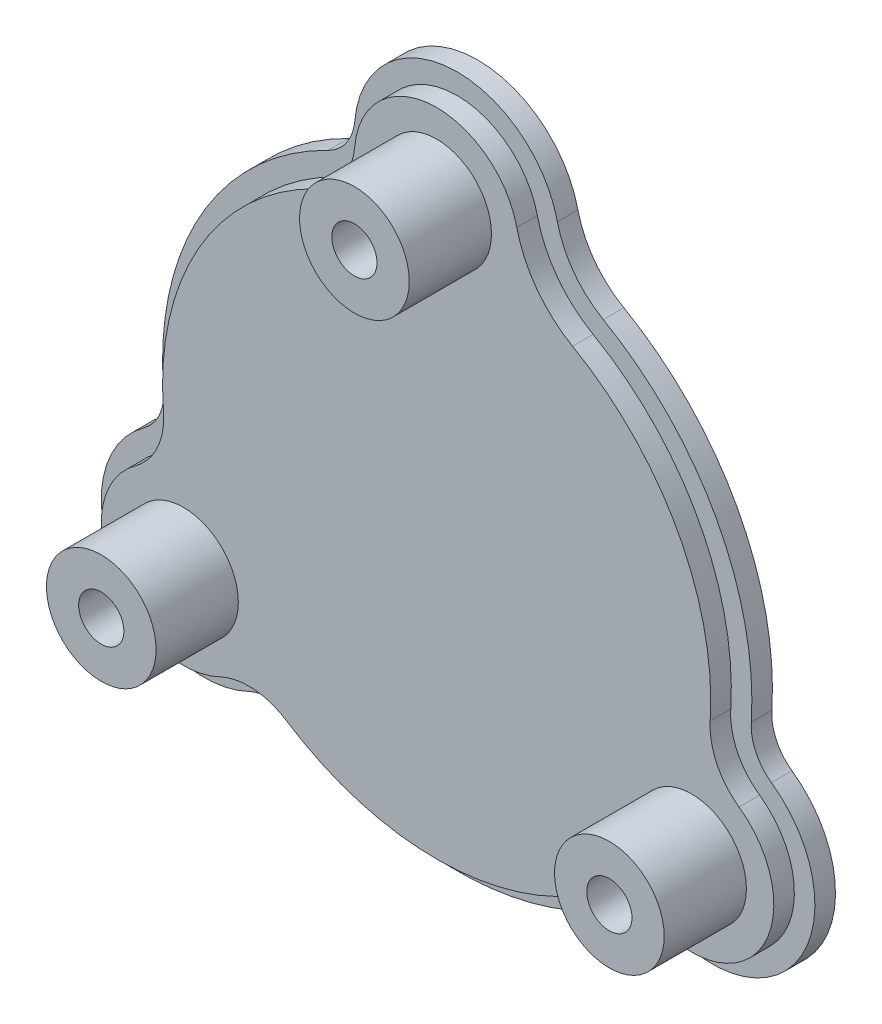
ISO-10303-21;
HEADER;
FILE_DESCRIPTION(('STEP AP214'),'2;1');
FILE_NAME('part.step','',(''),(''),'','','');
FILE_SCHEMA(('AUTOMOTIVE_DESIGN { 1 0 10303 214 1 1 1 1 }'));
ENDSEC;
DATA;
#1=APPLICATION_CONTEXT('core data for automotive mechanical design processes');
#2=APPLICATION_PROTOCOL_DEFINITION('international standard','automotive_design',2000,#1);
#3=PRODUCT_CONTEXT('',#1,'mechanical');
#4=PRODUCT('Part','Part','',(#3));
#5=PRODUCT_RELATED_PRODUCT_CATEGORY('part','',(#4));
#6=PRODUCT_DEFINITION_FORMATION('','',#4);
#7=PRODUCT_DEFINITION_CONTEXT('part definition',#1,'design');
#8=PRODUCT_DEFINITION('design','',#6,#7);
#9=PRODUCT_DEFINITION_SHAPE('','',#8);
#10=(LENGTH_UNIT() NAMED_UNIT(*) SI_UNIT(.MILLI.,.METRE.));
#11=(NAMED_UNIT(*) PLANE_ANGLE_UNIT() SI_UNIT($,.RADIAN.));
#12=(NAMED_UNIT(*) SI_UNIT($,.STERADIAN.) SOLID_ANGLE_UNIT());
#13=UNCERTAINTY_MEASURE_WITH_UNIT(LENGTH_MEASURE(1.E-05),#10,'distance_accuracy_value','');
#14=(GEOMETRIC_REPRESENTATION_CONTEXT(3) GLOBAL_UNCERTAINTY_ASSIGNED_CONTEXT((#13)) GLOBAL_UNIT_ASSIGNED_CONTEXT((#10,
#11,#12)) REPRESENTATION_CONTEXT('',''));
#15=CARTESIAN_POINT('',(0.,0.,0.));
#16=DIRECTION('',(0.,0.,1.));
#17=DIRECTION('',(1.,0.,0.));
#18=AXIS2_PLACEMENT_3D('',#15,#16,#17);
#19=CARTESIAN_POINT('',(-24.9125692180884,-2.08899376589599,3.));
#20=DIRECTION('',(0.,0.,1.));
#21=DIRECTION('',(1.,0.,0.));
#22=AXIS2_PLACEMENT_3D('',#19,#20,#21);
#23=PLANE('',#22);
#24=CARTESIAN_POINT('',(0.,0.,3.));
#25=DIRECTION('',(0.,0.,1.));
#26=DIRECTION('',(1.,0.,0.));
#27=AXIS2_PLACEMENT_3D('',#24,#25,#26);
#28=CIRCLE('',#27,43.);
#29=CARTESIAN_POINT('',(-18.8461534536892,38.65,3.));
#30=VERTEX_POINT('',#29);
#31=CARTESIAN_POINT('',(-42.8496190551121,-3.5930692773411,3.));
#32=VERTEX_POINT('',#31);
#33=EDGE_CURVE('E304',#30,#32,#28,.T.);
#34=ORIENTED_EDGE('',*,*,#33,.T.);
#35=CARTESIAN_POINT('',(-49.8251384361769,-4.17798753179198,3.));
#36=DIRECTION('',(0.,0.,-1.));
#37=DIRECTION('',(1.,0.,0.));
#38=AXIS2_PLACEMENT_3D('',#35,#36,#37);
#39=CIRCLE('',#38,7.);
#40=CARTESIAN_POINT('',(-45.7253382472528,-9.85175509936979,3.));
#41=VERTEX_POINT('',#40);
#42=EDGE_CURVE('E307',#32,#41,#39,.T.);
#43=ORIENTED_EDGE('',*,*,#42,.T.);
#44=CARTESIAN_POINT('',(-36.9400521281297,-22.0098284584651,3.));
#45=DIRECTION('',(0.,0.,1.));
#46=DIRECTION('',(1.,0.,0.));
#47=AXIS2_PLACEMENT_3D('',#44,#45,#46);
#48=CIRCLE('',#47,15.);
#49=CARTESIAN_POINT('',(-30.4295786984448,-35.5232934368253,3.));
#50=VERTEX_POINT('',#49);
#51=EDGE_CURVE('E309',#41,#50,#48,.T.);
#52=ORIENTED_EDGE('',*,*,#51,.T.);
#53=CARTESIAN_POINT('',(-27.3913577645918,-41.8295770933933,3.));
#54=DIRECTION('',(0.,0.,-1.));
#55=DIRECTION('',(1.,0.,0.));
#56=AXIS2_PLACEMENT_3D('',#53,#54,#55);
#57=CIRCLE('',#56,7.);
#58=CARTESIAN_POINT('',(-23.5565676775489,-35.9734363003183,3.));
#59=VERTEX_POINT('',#58);
#60=EDGE_CURVE('E315',#50,#59,#57,.T.);
#61=ORIENTED_EDGE('',*,*,#60,.T.);
#62=CARTESIAN_POINT('',(0.,0.,3.));
#63=DIRECTION('',(0.,0.,1.));
#64=DIRECTION('',(1.,0.,0.));
#65=AXIS2_PLACEMENT_3D('',#62,#63,#64);
#66=CIRCLE('',#65,43.);
#67=CARTESIAN_POINT('',(24.2998040125074,-35.4756187395474,3.));
#68=VERTEX_POINT('',#67);
#69=EDGE_CURVE('E314',#59,#68,#66,.T.);
#70=ORIENTED_EDGE('',*,*,#69,.T.);
#71=CARTESIAN_POINT('',(28.2555860610551,-41.25071946459,3.));
#72=DIRECTION('',(0.,0.,-1.));
#73=DIRECTION('',(1.,0.,0.));
#74=AXIS2_PLACEMENT_3D('',#71,#72,#73);
#75=CIRCLE('',#74,7.);
#76=CARTESIAN_POINT('',(31.1024364652992,-34.8557649865772,3.));
#77=VERTEX_POINT('',#76);
#78=EDGE_CURVE('E316',#68,#77,#75,.T.);
#79=ORIENTED_EDGE('',*,*,#78,.T.);
#80=CARTESIAN_POINT('',(37.2028301886792,-21.1522911051213,3.));
#81=DIRECTION('',(0.,0.,1.));
#82=DIRECTION('',(1.,0.,0.));
#83=AXIS2_PLACEMENT_3D('',#80,#81,#82);
#84=CIRCLE('',#83,15.);
#85=CARTESIAN_POINT('',(45.8589349502842,-8.90190946387765,3.));
#86=VERTEX_POINT('',#85);
#87=EDGE_CURVE('E318',#77,#86,#84,.T.);
#88=ORIENTED_EDGE('',*,*,#87,.T.);
#89=CARTESIAN_POINT('',(49.8984505056999,-3.18506469796396,3.));
#90=DIRECTION('',(0.,0.,-1.));
#91=DIRECTION('',(1.,0.,0.));
#92=AXIS2_PLACEMENT_3D('',#89,#90,#91);
#93=CIRCLE('',#92,7.);
#94=CARTESIAN_POINT('',(42.9126674349019,-2.739155640249,3.));
#95=VERTEX_POINT('',#94);
#96=EDGE_CURVE('E319',#86,#95,#93,.T.);
#97=ORIENTED_EDGE('',*,*,#96,.T.);
#98=CARTESIAN_POINT('',(0.,0.,3.));
#99=DIRECTION('',(0.,0.,1.));
#100=DIRECTION('',(1.,0.,0.));
#101=AXIS2_PLACEMENT_3D('',#98,#99,#100);
#102=CIRCLE('',#101,43.);
#103=CARTESIAN_POINT('',(21.320581007919,37.3421052631579,3.));
#104=VERTEX_POINT('',#103);
#105=EDGE_CURVE('E325',#95,#104,#102,.T.);
#106=ORIENTED_EDGE('',*,*,#105,.T.);
#107=CARTESIAN_POINT('',(28.2621655221252,49.5,3.));
#108=DIRECTION('',(0.,0.,-1.));
#109=DIRECTION('',(1.,0.,0.));
#110=AXIS2_PLACEMENT_3D('',#107,#108,#109);
#111=CIRCLE('',#110,14.);
#112=CARTESIAN_POINT('',(14.6183614769613,46.3620689655173,3.));
#113=VERTEX_POINT('',#112);
#114=EDGE_CURVE('E322',#104,#113,#111,.T.);
#115=ORIENTED_EDGE('',*,*,#114,.T.);
#116=CARTESIAN_POINT('',(0.,43.,3.));
#117=DIRECTION('',(0.,0.,1.));
#118=DIRECTION('',(1.,0.,0.));
#119=AXIS2_PLACEMENT_3D('',#116,#117,#118);
#120=CIRCLE('',#119,15.);
#121=CARTESIAN_POINT('',(-14.9414535837916,44.3239957716702,3.));
#122=VERTEX_POINT('',#121);
#123=EDGE_CURVE('E326',#113,#122,#120,.T.);
#124=ORIENTED_EDGE('',*,*,#123,.T.);
#125=CARTESIAN_POINT('',(-21.9141319228944,44.9418604651163,3.));
#126=DIRECTION('',(0.,0.,-1.));
#127=DIRECTION('',(1.,0.,0.));
#128=AXIS2_PLACEMENT_3D('',#125,#126,#127);
#129=CIRCLE('',#128,7.);
#130=EDGE_CURVE('E327',#122,#30,#129,.T.);
#131=ORIENTED_EDGE('',*,*,#130,.T.);
#132=EDGE_LOOP('',(#34,#43,#52,#61,#70,#79,#88,#97,#106,#115,#124,#131));
#133=FACE_BOUND('',#132,.T.);
#134=CARTESIAN_POINT('',(0.,0.,3.));
#135=DIRECTION('',(0.,0.,1.));
#136=DIRECTION('',(1.,0.,0.));
#137=AXIS2_PLACEMENT_3D('',#134,#135,#136);
#138=CIRCLE('',#137,40.);
#139=CARTESIAN_POINT('',(-17.5313055383155,35.953488372093,3.));
#140=VERTEX_POINT('',#139);
#141=CARTESIAN_POINT('',(-39.8601107489415,-3.34239002543356,3.));
#142=VERTEX_POINT('',#141);
#143=EDGE_CURVE('E218',#140,#142,#138,.T.);
#144=ORIENTED_EDGE('',*,*,#143,.F.);
#145=CARTESIAN_POINT('',(-21.9141319228944,44.9418604651163,3.));
#146=DIRECTION('',(0.,0.,1.));
#147=DIRECTION('',(1.,0.,0.));
#148=AXIS2_PLACEMENT_3D('',#145,#146,#147);
#149=CIRCLE('',#148,10.);
#150=CARTESIAN_POINT('',(-11.9531628670333,44.0591966173361,3.));
#151=VERTEX_POINT('',#150);
#152=EDGE_CURVE('E53',#140,#151,#149,.T.);
#153=ORIENTED_EDGE('',*,*,#152,.T.);
#154=CARTESIAN_POINT('',(0.,43.,3.));
#155=DIRECTION('',(0.,0.,1.));
#156=DIRECTION('',(1.,0.,0.));
#157=AXIS2_PLACEMENT_3D('',#154,#155,#156);
#158=CIRCLE('',#157,12.);
#159=CARTESIAN_POINT('',(11.694689181569,45.6896551724138,3.));
#160=VERTEX_POINT('',#159);
#161=EDGE_CURVE('E56',#160,#151,#158,.T.);
#162=ORIENTED_EDGE('',*,*,#161,.F.);
#163=CARTESIAN_POINT('',(28.2621655221252,49.5,3.));
#164=DIRECTION('',(0.,0.,1.));
#165=DIRECTION('',(1.,0.,0.));
#166=AXIS2_PLACEMENT_3D('',#163,#164,#165);
#167=CIRCLE('',#166,17.);
#168=CARTESIAN_POINT('',(19.8330986120176,34.7368421052632,3.));
#169=VERTEX_POINT('',#168);
#170=EDGE_CURVE('E251',#160,#169,#167,.T.);
#171=ORIENTED_EDGE('',*,*,#170,.T.);
#172=CARTESIAN_POINT('',(0.,0.,3.));
#173=DIRECTION('',(0.,0.,1.));
#174=DIRECTION('',(1.,0.,0.));
#175=AXIS2_PLACEMENT_3D('',#172,#173,#174);
#176=CIRCLE('',#175,40.);
#177=CARTESIAN_POINT('',(39.9187604045599,-2.54805175837117,3.));
#178=VERTEX_POINT('',#177);
#179=EDGE_CURVE('E254',#178,#169,#176,.T.);
#180=ORIENTED_EDGE('',*,*,#179,.F.);
#181=CARTESIAN_POINT('',(49.8984505056999,-3.18506469796396,3.));
#182=DIRECTION('',(0.,0.,1.));
#183=DIRECTION('',(1.,0.,0.));
#184=AXIS2_PLACEMENT_3D('',#181,#182,#183);
#185=CIRCLE('',#184,10.);
#186=CARTESIAN_POINT('',(44.1277139979632,-11.3519857921264,3.));
#187=VERTEX_POINT('',#186);
#188=EDGE_CURVE('E256',#178,#187,#185,.T.);
#189=ORIENTED_EDGE('',*,*,#188,.T.);
#190=CARTESIAN_POINT('',(37.2028301886792,-21.1522911051213,3.));
#191=DIRECTION('',(0.,0.,1.));
#192=DIRECTION('',(1.,0.,0.));
#193=AXIS2_PLACEMENT_3D('',#190,#191,#192);
#194=CIRCLE('',#193,12.);
#195=CARTESIAN_POINT('',(32.3225152099752,-32.115070210286,3.));
#196=VERTEX_POINT('',#195);
#197=EDGE_CURVE('E257',#196,#187,#194,.T.);
#198=ORIENTED_EDGE('',*,*,#197,.F.);
#199=CARTESIAN_POINT('',(28.2555860610551,-41.25071946459,3.));
#200=DIRECTION('',(0.,0.,1.));
#201=DIRECTION('',(1.,0.,0.));
#202=AXIS2_PLACEMENT_3D('',#199,#200,#201);
#203=CIRCLE('',#202,9.99999999999999);
#204=CARTESIAN_POINT('',(22.6044688488441,-33.000575571672,3.));
#205=VERTEX_POINT('',#204);
#206=EDGE_CURVE('E263',#196,#205,#203,.T.);
#207=ORIENTED_EDGE('',*,*,#206,.T.);
#208=CARTESIAN_POINT('',(0.,0.,3.));
#209=DIRECTION('',(0.,0.,1.));
#210=DIRECTION('',(1.,0.,0.));
#211=AXIS2_PLACEMENT_3D('',#208,#209,#210);
#212=CIRCLE('',#211,40.);
#213=CARTESIAN_POINT('',(-21.9130862116734,-33.4636616747147,3.));
#214=VERTEX_POINT('',#213);
#215=EDGE_CURVE('E264',#214,#205,#212,.T.);
#216=ORIENTED_EDGE('',*,*,#215,.F.);
#217=CARTESIAN_POINT('',(-27.3913577645918,-41.8295770933933,3.));
#218=DIRECTION('',(0.,0.,1.));
#219=DIRECTION('',(1.,0.,0.));
#220=AXIS2_PLACEMENT_3D('',#217,#218,#219);
#221=CIRCLE('',#220,10.);
#222=CARTESIAN_POINT('',(-31.7316733843817,-32.8206004411532,3.));
#223=VERTEX_POINT('',#222);
#224=EDGE_CURVE('E268',#214,#223,#221,.T.);
#225=ORIENTED_EDGE('',*,*,#224,.T.);
#226=CARTESIAN_POINT('',(-36.9400521281297,-22.0098284584651,3.));
#227=DIRECTION('',(0.,0.,1.));
#228=DIRECTION('',(1.,0.,0.));
#229=AXIS2_PLACEMENT_3D('',#226,#227,#228);
#230=CIRCLE('',#229,12.);
#231=CARTESIAN_POINT('',(-43.9682810234281,-12.2833697711889,3.));
#232=VERTEX_POINT('',#231);
#233=EDGE_CURVE('E269',#232,#223,#230,.T.);
#234=ORIENTED_EDGE('',*,*,#233,.F.);
#235=CARTESIAN_POINT('',(-49.8251384361769,-4.17798753179198,3.));
#236=DIRECTION('',(0.,0.,1.));
#237=DIRECTION('',(1.,0.,0.));
#238=AXIS2_PLACEMENT_3D('',#235,#236,#237);
#239=CIRCLE('',#238,10.);
#240=EDGE_CURVE('E225',#232,#142,#239,.T.);
#241=ORIENTED_EDGE('',*,*,#240,.T.);
#242=EDGE_LOOP('',(#144,#153,#162,#171,#180,#189,#198,#207,#216,#225,#234,#241));
#243=FACE_BOUND('',#242,.T.);
#244=ADVANCED_FACE('F39',(#133,#243),#23,.T.);
#245=CARTESIAN_POINT('',(0.,0.,3.));
#246=DIRECTION('',(0.,0.,-1.));
#247=DIRECTION('',(-1.,0.,0.));
#248=AXIS2_PLACEMENT_3D('',#245,#246,#247);
#249=CYLINDRICAL_SURFACE('',#248,43.);
#250=CARTESIAN_POINT('',(0.,0.,0.));
#251=DIRECTION('',(0.,0.,1.));
#252=DIRECTION('',(1.,0.,0.));
#253=AXIS2_PLACEMENT_3D('',#250,#251,#252);
#254=CIRCLE('',#253,43.);
#255=CARTESIAN_POINT('',(-18.8461534536892,38.65,0.));
#256=VERTEX_POINT('',#255);
#257=CARTESIAN_POINT('',(-42.8496190551121,-3.5930692773411,0.));
#258=VERTEX_POINT('',#257);
#259=EDGE_CURVE('E274',#256,#258,#254,.T.);
#260=ORIENTED_EDGE('',*,*,#259,.T.);
#261=DIRECTION('',(0.,0.,-1.));
#262=VECTOR('',#261,1.);
#263=CARTESIAN_POINT('',(-42.8496190551121,-3.5930692773411,3.));
#264=LINE('',#263,#262);
#265=EDGE_CURVE('E11',#32,#258,#264,.T.);
#266=ORIENTED_EDGE('',*,*,#265,.F.);
#267=ORIENTED_EDGE('',*,*,#33,.F.);
#268=DIRECTION('',(0.,0.,-1.));
#269=VECTOR('',#268,1.);
#270=CARTESIAN_POINT('',(-18.8461534536892,38.65,3.));
#271=LINE('',#270,#269);
#272=EDGE_CURVE('E329',#30,#256,#271,.T.);
#273=ORIENTED_EDGE('',*,*,#272,.T.);
#274=EDGE_LOOP('',(#260,#266,#267,#273));
#275=FACE_BOUND('',#274,.T.);
#276=ADVANCED_FACE('F41',(#275),#249,.T.);
#277=CARTESIAN_POINT('',(-49.8251384361769,-4.17798753179198,3.));
#278=DIRECTION('',(0.,0.,-1.));
#279=DIRECTION('',(-1.,0.,0.));
#280=AXIS2_PLACEMENT_3D('',#277,#278,#279);
#281=CYLINDRICAL_SURFACE('',#280,7.);
#282=CARTESIAN_POINT('',(-49.8251384361769,-4.17798753179198,0.));
#283=DIRECTION('',(0.,0.,-1.));
#284=DIRECTION('',(1.,0.,0.));
#285=AXIS2_PLACEMENT_3D('',#282,#283,#284);
#286=CIRCLE('',#285,7.);
#287=CARTESIAN_POINT('',(-45.7253382472528,-9.85175509936979,0.));
#288=VERTEX_POINT('',#287);
#289=EDGE_CURVE('E334',#258,#288,#286,.T.);
#290=ORIENTED_EDGE('',*,*,#289,.T.);
#291=DIRECTION('',(0.,0.,-1.));
#292=VECTOR('',#291,1.);
#293=CARTESIAN_POINT('',(-45.7253382472528,-9.85175509936979,3.));
#294=LINE('',#293,#292);
#295=EDGE_CURVE('E50',#41,#288,#294,.T.);
#296=ORIENTED_EDGE('',*,*,#295,.F.);
#297=ORIENTED_EDGE('',*,*,#42,.F.);
#298=ORIENTED_EDGE('',*,*,#265,.T.);
#299=EDGE_LOOP('',(#290,#296,#297,#298));
#300=FACE_BOUND('',#299,.T.);
#301=ADVANCED_FACE('F408',(#300),#281,.F.);
#302=CARTESIAN_POINT('',(-36.9400521281297,-22.0098284584651,3.));
#303=DIRECTION('',(0.,0.,-1.));
#304=DIRECTION('',(-1.,0.,0.));
#305=AXIS2_PLACEMENT_3D('',#302,#303,#304);
#306=CYLINDRICAL_SURFACE('',#305,15.);
#307=CARTESIAN_POINT('',(-36.9400521281297,-22.0098284584651,0.));
#308=DIRECTION('',(0.,0.,1.));
#309=DIRECTION('',(1.,0.,0.));
#310=AXIS2_PLACEMENT_3D('',#307,#308,#309);
#311=CIRCLE('',#310,15.);
#312=CARTESIAN_POINT('',(-30.4295786984448,-35.5232934368253,0.));
#313=VERTEX_POINT('',#312);
#314=EDGE_CURVE('E333',#288,#313,#311,.T.);
#315=ORIENTED_EDGE('',*,*,#314,.T.);
#316=DIRECTION('',(0.,0.,-1.));
#317=VECTOR('',#316,1.);
#318=CARTESIAN_POINT('',(-30.4295786984448,-35.5232934368253,3.));
#319=LINE('',#318,#317);
#320=EDGE_CURVE('E379',#50,#313,#319,.T.);
#321=ORIENTED_EDGE('',*,*,#320,.F.);
#322=ORIENTED_EDGE('',*,*,#51,.F.);
#323=ORIENTED_EDGE('',*,*,#295,.T.);
#324=EDGE_LOOP('',(#315,#321,#322,#323));
#325=FACE_BOUND('',#324,.T.);
#326=ADVANCED_FACE('F390',(#325),#306,.T.);
#327=CARTESIAN_POINT('',(-27.3913577645918,-41.8295770933933,3.));
#328=DIRECTION('',(0.,0.,-1.));
#329=DIRECTION('',(-1.,0.,0.));
#330=AXIS2_PLACEMENT_3D('',#327,#328,#329);
#331=CYLINDRICAL_SURFACE('',#330,7.);
#332=CARTESIAN_POINT('',(-27.3913577645918,-41.8295770933933,0.));
#333=DIRECTION('',(0.,0.,-1.));
#334=DIRECTION('',(1.,0.,0.));
#335=AXIS2_PLACEMENT_3D('',#332,#333,#334);
#336=CIRCLE('',#335,7.);
#337=CARTESIAN_POINT('',(-23.5565676775489,-35.9734363003183,0.));
#338=VERTEX_POINT('',#337);
#339=EDGE_CURVE('E336',#313,#338,#336,.T.);
#340=ORIENTED_EDGE('',*,*,#339,.T.);
#341=DIRECTION('',(0.,0.,-1.));
#342=VECTOR('',#341,1.);
#343=CARTESIAN_POINT('',(-23.5565676775489,-35.9734363003183,3.));
#344=LINE('',#343,#342);
#345=EDGE_CURVE('E380',#59,#338,#344,.T.);
#346=ORIENTED_EDGE('',*,*,#345,.F.);
#347=ORIENTED_EDGE('',*,*,#60,.F.);
#348=ORIENTED_EDGE('',*,*,#320,.T.);
#349=EDGE_LOOP('',(#340,#346,#347,#348));
#350=FACE_BOUND('',#349,.T.);
#351=ADVANCED_FACE('F396',(#350),#331,.F.);
#352=CARTESIAN_POINT('',(0.,0.,3.));
#353=DIRECTION('',(0.,0.,-1.));
#354=DIRECTION('',(-1.,0.,0.));
#355=AXIS2_PLACEMENT_3D('',#352,#353,#354);
#356=CYLINDRICAL_SURFACE('',#355,43.);
#357=CARTESIAN_POINT('',(0.,0.,0.));
#358=DIRECTION('',(0.,0.,1.));
#359=DIRECTION('',(1.,0.,0.));
#360=AXIS2_PLACEMENT_3D('',#357,#358,#359);
#361=CIRCLE('',#360,43.);
#362=CARTESIAN_POINT('',(24.2998040125074,-35.4756187395474,0.));
#363=VERTEX_POINT('',#362);
#364=EDGE_CURVE('E338',#338,#363,#361,.T.);
#365=ORIENTED_EDGE('',*,*,#364,.T.);
#366=DIRECTION('',(0.,0.,-1.));
#367=VECTOR('',#366,1.);
#368=CARTESIAN_POINT('',(24.2998040125074,-35.4756187395474,3.));
#369=LINE('',#368,#367);
#370=EDGE_CURVE('E372',#68,#363,#369,.T.);
#371=ORIENTED_EDGE('',*,*,#370,.F.);
#372=ORIENTED_EDGE('',*,*,#69,.F.);
#373=ORIENTED_EDGE('',*,*,#345,.T.);
#374=EDGE_LOOP('',(#365,#371,#372,#373));
#375=FACE_BOUND('',#374,.T.);
#376=ADVANCED_FACE('F405',(#375),#356,.T.);
#377=CARTESIAN_POINT('',(28.2555860610551,-41.25071946459,3.));
#378=DIRECTION('',(0.,0.,-1.));
#379=DIRECTION('',(-1.,0.,0.));
#380=AXIS2_PLACEMENT_3D('',#377,#378,#379);
#381=CYLINDRICAL_SURFACE('',#380,7.);
#382=CARTESIAN_POINT('',(28.2555860610551,-41.25071946459,0.));
#383=DIRECTION('',(0.,0.,-1.));
#384=DIRECTION('',(1.,0.,0.));
#385=AXIS2_PLACEMENT_3D('',#382,#383,#384);
#386=CIRCLE('',#385,7.);
#387=CARTESIAN_POINT('',(31.1024364652992,-34.8557649865772,0.));
#388=VERTEX_POINT('',#387);
#389=EDGE_CURVE('E343',#363,#388,#386,.T.);
#390=ORIENTED_EDGE('',*,*,#389,.T.);
#391=DIRECTION('',(0.,0.,-1.));
#392=VECTOR('',#391,1.);
#393=CARTESIAN_POINT('',(31.1024364652992,-34.8557649865772,3.));
#394=LINE('',#393,#392);
#395=EDGE_CURVE('E371',#77,#388,#394,.T.);
#396=ORIENTED_EDGE('',*,*,#395,.F.);
#397=ORIENTED_EDGE('',*,*,#78,.F.);
#398=ORIENTED_EDGE('',*,*,#370,.T.);
#399=EDGE_LOOP('',(#390,#396,#397,#398));
#400=FACE_BOUND('',#399,.T.);
#401=ADVANCED_FACE('F445',(#400),#381,.F.);
#402=CARTESIAN_POINT('',(37.2028301886792,-21.1522911051213,3.));
#403=DIRECTION('',(0.,0.,-1.));
#404=DIRECTION('',(-1.,0.,0.));
#405=AXIS2_PLACEMENT_3D('',#402,#403,#404);
#406=CYLINDRICAL_SURFACE('',#405,15.);
#407=CARTESIAN_POINT('',(37.2028301886792,-21.1522911051213,0.));
#408=DIRECTION('',(0.,0.,1.));
#409=DIRECTION('',(1.,0.,0.));
#410=AXIS2_PLACEMENT_3D('',#407,#408,#409);
#411=CIRCLE('',#410,15.);
#412=CARTESIAN_POINT('',(45.8589349502842,-8.90190946387765,0.));
#413=VERTEX_POINT('',#412);
#414=EDGE_CURVE('E341',#388,#413,#411,.T.);
#415=ORIENTED_EDGE('',*,*,#414,.T.);
#416=DIRECTION('',(0.,0.,-1.));
#417=VECTOR('',#416,1.);
#418=CARTESIAN_POINT('',(45.8589349502842,-8.90190946387765,3.));
#419=LINE('',#418,#417);
#420=EDGE_CURVE('E366',#86,#413,#419,.T.);
#421=ORIENTED_EDGE('',*,*,#420,.F.);
#422=ORIENTED_EDGE('',*,*,#87,.F.);
#423=ORIENTED_EDGE('',*,*,#395,.T.);
#424=EDGE_LOOP('',(#415,#421,#422,#423));
#425=FACE_BOUND('',#424,.T.);
#426=ADVANCED_FACE('F439',(#425),#406,.T.);
#427=CARTESIAN_POINT('',(49.8984505056999,-3.18506469796396,3.));
#428=DIRECTION('',(0.,0.,-1.));
#429=DIRECTION('',(-1.,0.,0.));
#430=AXIS2_PLACEMENT_3D('',#427,#428,#429);
#431=CYLINDRICAL_SURFACE('',#430,7.);
#432=CARTESIAN_POINT('',(49.8984505056999,-3.18506469796396,0.));
#433=DIRECTION('',(0.,0.,-1.));
#434=DIRECTION('',(1.,0.,0.));
#435=AXIS2_PLACEMENT_3D('',#432,#433,#434);
#436=CIRCLE('',#435,7.);
#437=CARTESIAN_POINT('',(42.9126674349019,-2.739155640249,0.));
#438=VERTEX_POINT('',#437);
#439=EDGE_CURVE('E342',#413,#438,#436,.T.);
#440=ORIENTED_EDGE('',*,*,#439,.T.);
#441=DIRECTION('',(0.,0.,-1.));
#442=VECTOR('',#441,1.);
#443=CARTESIAN_POINT('',(42.9126674349019,-2.739155640249,3.));
#444=LINE('',#443,#442);
#445=EDGE_CURVE('E364',#95,#438,#444,.T.);
#446=ORIENTED_EDGE('',*,*,#445,.F.);
#447=ORIENTED_EDGE('',*,*,#96,.F.);
#448=ORIENTED_EDGE('',*,*,#420,.T.);
#449=EDGE_LOOP('',(#440,#446,#447,#448));
#450=FACE_BOUND('',#449,.T.);
#451=ADVANCED_FACE('F436',(#450),#431,.F.);
#452=CARTESIAN_POINT('',(0.,0.,3.));
#453=DIRECTION('',(0.,0.,-1.));
#454=DIRECTION('',(-1.,0.,0.));
#455=AXIS2_PLACEMENT_3D('',#452,#453,#454);
#456=CYLINDRICAL_SURFACE('',#455,43.);
#457=CARTESIAN_POINT('',(0.,0.,0.));
#458=DIRECTION('',(0.,0.,1.));
#459=DIRECTION('',(1.,0.,0.));
#460=AXIS2_PLACEMENT_3D('',#457,#458,#459);
#461=CIRCLE('',#460,43.);
#462=CARTESIAN_POINT('',(21.320581007919,37.3421052631579,0.));
#463=VERTEX_POINT('',#462);
#464=EDGE_CURVE('E350',#438,#463,#461,.T.);
#465=ORIENTED_EDGE('',*,*,#464,.T.);
#466=DIRECTION('',(0.,0.,-1.));
#467=VECTOR('',#466,1.);
#468=CARTESIAN_POINT('',(21.320581007919,37.3421052631579,3.));
#469=LINE('',#468,#467);
#470=EDGE_CURVE('E362',#104,#463,#469,.T.);
#471=ORIENTED_EDGE('',*,*,#470,.F.);
#472=ORIENTED_EDGE('',*,*,#105,.F.);
#473=ORIENTED_EDGE('',*,*,#445,.T.);
#474=EDGE_LOOP('',(#465,#471,#472,#473));
#475=FACE_BOUND('',#474,.T.);
#476=ADVANCED_FACE('F431',(#475),#456,.T.);
#477=CARTESIAN_POINT('',(28.2621655221252,49.5,3.));
#478=DIRECTION('',(0.,0.,-1.));
#479=DIRECTION('',(-1.,0.,0.));
#480=AXIS2_PLACEMENT_3D('',#477,#478,#479);
#481=CYLINDRICAL_SURFACE('',#480,14.);
#482=CARTESIAN_POINT('',(28.2621655221252,49.5,0.));
#483=DIRECTION('',(0.,0.,-1.));
#484=DIRECTION('',(1.,0.,0.));
#485=AXIS2_PLACEMENT_3D('',#482,#483,#484);
#486=CIRCLE('',#485,14.);
#487=CARTESIAN_POINT('',(14.6183614769613,46.3620689655173,0.));
#488=VERTEX_POINT('',#487);
#489=EDGE_CURVE('E349',#463,#488,#486,.T.);
#490=ORIENTED_EDGE('',*,*,#489,.T.);
#491=DIRECTION('',(0.,0.,-1.));
#492=VECTOR('',#491,1.);
#493=CARTESIAN_POINT('',(14.6183614769613,46.3620689655173,3.));
#494=LINE('',#493,#492);
#495=EDGE_CURVE('E359',#113,#488,#494,.T.);
#496=ORIENTED_EDGE('',*,*,#495,.F.);
#497=ORIENTED_EDGE('',*,*,#114,.F.);
#498=ORIENTED_EDGE('',*,*,#470,.T.);
#499=EDGE_LOOP('',(#490,#496,#497,#498));
#500=FACE_BOUND('',#499,.T.);
#501=ADVANCED_FACE('F422',(#500),#481,.F.);
#502=CARTESIAN_POINT('',(0.,43.,3.));
#503=DIRECTION('',(0.,0.,-1.));
#504=DIRECTION('',(-1.,0.,0.));
#505=AXIS2_PLACEMENT_3D('',#502,#503,#504);
#506=CYLINDRICAL_SURFACE('',#505,15.);
#507=CARTESIAN_POINT('',(0.,43.,0.));
#508=DIRECTION('',(0.,0.,1.));
#509=DIRECTION('',(1.,0.,0.));
#510=AXIS2_PLACEMENT_3D('',#507,#508,#509);
#511=CIRCLE('',#510,15.);
#512=CARTESIAN_POINT('',(-14.9414535837916,44.3239957716702,0.));
#513=VERTEX_POINT('',#512);
#514=EDGE_CURVE('E354',#488,#513,#511,.T.);
#515=ORIENTED_EDGE('',*,*,#514,.T.);
#516=DIRECTION('',(0.,0.,-1.));
#517=VECTOR('',#516,1.);
#518=CARTESIAN_POINT('',(-14.9414535837916,44.3239957716702,3.));
#519=LINE('',#518,#517);
#520=EDGE_CURVE('E358',#122,#513,#519,.T.);
#521=ORIENTED_EDGE('',*,*,#520,.F.);
#522=ORIENTED_EDGE('',*,*,#123,.F.);
#523=ORIENTED_EDGE('',*,*,#495,.T.);
#524=EDGE_LOOP('',(#515,#521,#522,#523));
#525=FACE_BOUND('',#524,.T.);
#526=ADVANCED_FACE('F423',(#525),#506,.T.);
#527=CARTESIAN_POINT('',(-21.9141319228944,44.9418604651163,3.));
#528=DIRECTION('',(0.,0.,-1.));
#529=DIRECTION('',(-1.,0.,0.));
#530=AXIS2_PLACEMENT_3D('',#527,#528,#529);
#531=CYLINDRICAL_SURFACE('',#530,7.);
#532=CARTESIAN_POINT('',(-21.9141319228944,44.9418604651163,0.));
#533=DIRECTION('',(0.,0.,-1.));
#534=DIRECTION('',(1.,0.,0.));
#535=AXIS2_PLACEMENT_3D('',#532,#533,#534);
#536=CIRCLE('',#535,7.);
#537=EDGE_CURVE('E306',#513,#256,#536,.T.);
#538=ORIENTED_EDGE('',*,*,#537,.T.);
#539=ORIENTED_EDGE('',*,*,#272,.F.);
#540=ORIENTED_EDGE('',*,*,#130,.F.);
#541=ORIENTED_EDGE('',*,*,#520,.T.);
#542=EDGE_LOOP('',(#538,#539,#540,#541));
#543=FACE_BOUND('',#542,.T.);
#544=ADVANCED_FACE('F418',(#543),#531,.F.);
#545=CARTESIAN_POINT('',(-24.9125692180884,-2.08899376589599,0.));
#546=DIRECTION('',(0.,0.,1.));
#547=DIRECTION('',(1.,0.,0.));
#548=AXIS2_PLACEMENT_3D('',#545,#546,#547);
#549=PLANE('',#548);
#550=CARTESIAN_POINT('',(0.,43.,0.));
#551=DIRECTION('',(0.,0.,1.));
#552=DIRECTION('',(1.,0.,0.));
#553=AXIS2_PLACEMENT_3D('',#550,#551,#552);
#554=CIRCLE('',#553,3.3);
#555=CARTESIAN_POINT('',(3.3,43.,0.));
#556=VERTEX_POINT('',#555);
#557=EDGE_CURVE('E726',#556,#556,#554,.T.);
#558=ORIENTED_EDGE('',*,*,#557,.T.);
#559=EDGE_LOOP('',(#558));
#560=FACE_BOUND('',#559,.T.);
#561=CARTESIAN_POINT('',(37.2028301886792,-21.1522911051213,0.));
#562=DIRECTION('',(0.,0.,1.));
#563=DIRECTION('',(1.,0.,0.));
#564=AXIS2_PLACEMENT_3D('',#561,#562,#563);
#565=CIRCLE('',#564,3.3);
#566=CARTESIAN_POINT('',(40.5028301886792,-21.1522911051213,0.));
#567=VERTEX_POINT('',#566);
#568=EDGE_CURVE('E727',#567,#567,#565,.T.);
#569=ORIENTED_EDGE('',*,*,#568,.T.);
#570=EDGE_LOOP('',(#569));
#571=FACE_BOUND('',#570,.T.);
#572=CARTESIAN_POINT('',(-36.9400521281297,-22.0098284584651,0.));
#573=DIRECTION('',(0.,0.,1.));
#574=DIRECTION('',(1.,0.,0.));
#575=AXIS2_PLACEMENT_3D('',#572,#573,#574);
#576=CIRCLE('',#575,3.3);
#577=CARTESIAN_POINT('',(-33.6400521281297,-22.0098284584651,0.));
#578=VERTEX_POINT('',#577);
#579=EDGE_CURVE('E739',#578,#578,#576,.T.);
#580=ORIENTED_EDGE('',*,*,#579,.T.);
#581=EDGE_LOOP('',(#580));
#582=FACE_BOUND('',#581,.T.);
#583=ORIENTED_EDGE('',*,*,#259,.F.);
#584=ORIENTED_EDGE('',*,*,#537,.F.);
#585=ORIENTED_EDGE('',*,*,#514,.F.);
#586=ORIENTED_EDGE('',*,*,#489,.F.);
#587=ORIENTED_EDGE('',*,*,#464,.F.);
#588=ORIENTED_EDGE('',*,*,#439,.F.);
#589=ORIENTED_EDGE('',*,*,#414,.F.);
#590=ORIENTED_EDGE('',*,*,#389,.F.);
#591=ORIENTED_EDGE('',*,*,#364,.F.);
#592=ORIENTED_EDGE('',*,*,#339,.F.);
#593=ORIENTED_EDGE('',*,*,#314,.F.);
#594=ORIENTED_EDGE('',*,*,#289,.F.);
#595=EDGE_LOOP('',(#583,#584,#585,#586,#587,#588,#589,#590,#591,#592,#593,#594));
#596=FACE_BOUND('',#595,.T.);
#597=ADVANCED_FACE('F395',(#560,#571,#582,#596),#549,.F.);
#598=CARTESIAN_POINT('',(-21.9141319228944,44.9418604651163,6.));
#599=DIRECTION('',(0.,0.,-1.));
#600=DIRECTION('',(-1.,0.,0.));
#601=AXIS2_PLACEMENT_3D('',#598,#599,#600);
#602=CYLINDRICAL_SURFACE('',#601,10.);
#603=ORIENTED_EDGE('',*,*,#152,.F.);
#604=DIRECTION('',(0.,0.,-1.));
#605=VECTOR('',#604,1.);
#606=CARTESIAN_POINT('',(-17.5313055383155,35.953488372093,6.));
#607=LINE('',#606,#605);
#608=CARTESIAN_POINT('',(-17.5313055383155,35.953488372093,6.));
#609=VERTEX_POINT('',#608);
#610=EDGE_CURVE('E220',#609,#140,#607,.T.);
#611=ORIENTED_EDGE('',*,*,#610,.F.);
#612=CARTESIAN_POINT('',(-21.9141319228944,44.9418604651163,6.));
#613=DIRECTION('',(0.,0.,1.));
#614=DIRECTION('',(1.,0.,0.));
#615=AXIS2_PLACEMENT_3D('',#612,#613,#614);
#616=CIRCLE('',#615,10.);
#617=CARTESIAN_POINT('',(-11.9531628670333,44.0591966173361,6.));
#618=VERTEX_POINT('',#617);
#619=EDGE_CURVE('E204',#609,#618,#616,.T.);
#620=ORIENTED_EDGE('',*,*,#619,.T.);
#621=DIRECTION('',(0.,0.,-1.));
#622=VECTOR('',#621,1.);
#623=CARTESIAN_POINT('',(-11.9531628670333,44.0591966173361,6.));
#624=LINE('',#623,#622);
#625=EDGE_CURVE('E207',#618,#151,#624,.T.);
#626=ORIENTED_EDGE('',*,*,#625,.T.);
#627=EDGE_LOOP('',(#603,#611,#620,#626));
#628=FACE_BOUND('',#627,.T.);
#629=ADVANCED_FACE('F214',(#628),#602,.F.);
#630=CARTESIAN_POINT('',(0.,0.,6.));
#631=DIRECTION('',(0.,0.,-1.));
#632=DIRECTION('',(-1.,0.,0.));
#633=AXIS2_PLACEMENT_3D('',#630,#631,#632);
#634=CYLINDRICAL_SURFACE('',#633,40.);
#635=ORIENTED_EDGE('',*,*,#143,.T.);
#636=DIRECTION('',(0.,0.,-1.));
#637=VECTOR('',#636,1.);
#638=CARTESIAN_POINT('',(-39.8601107489415,-3.34239002543356,6.));
#639=LINE('',#638,#637);
#640=CARTESIAN_POINT('',(-39.8601107489415,-3.34239002543356,6.));
#641=VERTEX_POINT('',#640);
#642=EDGE_CURVE('E277',#641,#142,#639,.T.);
#643=ORIENTED_EDGE('',*,*,#642,.F.);
#644=CARTESIAN_POINT('',(0.,0.,6.));
#645=DIRECTION('',(0.,0.,1.));
#646=DIRECTION('',(1.,0.,0.));
#647=AXIS2_PLACEMENT_3D('',#644,#645,#646);
#648=CIRCLE('',#647,40.);
#649=EDGE_CURVE('E213',#609,#641,#648,.T.);
#650=ORIENTED_EDGE('',*,*,#649,.F.);
#651=ORIENTED_EDGE('',*,*,#610,.T.);
#652=EDGE_LOOP('',(#635,#643,#650,#651));
#653=FACE_BOUND('',#652,.T.);
#654=ADVANCED_FACE('F516',(#653),#634,.T.);
#655=CARTESIAN_POINT('',(-49.8251384361769,-4.17798753179198,6.));
#656=DIRECTION('',(0.,0.,-1.));
#657=DIRECTION('',(-1.,0.,0.));
#658=AXIS2_PLACEMENT_3D('',#655,#656,#657);
#659=CYLINDRICAL_SURFACE('',#658,10.);
#660=ORIENTED_EDGE('',*,*,#240,.F.);
#661=DIRECTION('',(0.,0.,-1.));
#662=VECTOR('',#661,1.);
#663=CARTESIAN_POINT('',(-43.9682810234281,-12.2833697711889,6.));
#664=LINE('',#663,#662);
#665=CARTESIAN_POINT('',(-43.9682810234281,-12.2833697711889,6.));
#666=VERTEX_POINT('',#665);
#667=EDGE_CURVE('E276',#666,#232,#664,.T.);
#668=ORIENTED_EDGE('',*,*,#667,.F.);
#669=CARTESIAN_POINT('',(-49.8251384361769,-4.17798753179198,6.));
#670=DIRECTION('',(0.,0.,1.));
#671=DIRECTION('',(1.,0.,0.));
#672=AXIS2_PLACEMENT_3D('',#669,#670,#671);
#673=CIRCLE('',#672,10.);
#674=EDGE_CURVE('E248',#666,#641,#673,.T.);
#675=ORIENTED_EDGE('',*,*,#674,.T.);
#676=ORIENTED_EDGE('',*,*,#642,.T.);
#677=EDGE_LOOP('',(#660,#668,#675,#676));
#678=FACE_BOUND('',#677,.T.);
#679=ADVANCED_FACE('F522',(#678),#659,.F.);
#680=CARTESIAN_POINT('',(-36.9400521281297,-22.0098284584651,6.));
#681=DIRECTION('',(0.,0.,-1.));
#682=DIRECTION('',(-1.,0.,0.));
#683=AXIS2_PLACEMENT_3D('',#680,#681,#682);
#684=CYLINDRICAL_SURFACE('',#683,12.);
#685=ORIENTED_EDGE('',*,*,#233,.T.);
#686=DIRECTION('',(0.,0.,-1.));
#687=VECTOR('',#686,1.);
#688=CARTESIAN_POINT('',(-31.7316733843817,-32.8206004411532,6.));
#689=LINE('',#688,#687);
#690=CARTESIAN_POINT('',(-31.7316733843817,-32.8206004411532,6.));
#691=VERTEX_POINT('',#690);
#692=EDGE_CURVE('E281',#691,#223,#689,.T.);
#693=ORIENTED_EDGE('',*,*,#692,.F.);
#694=CARTESIAN_POINT('',(-36.9400521281297,-22.0098284584651,6.));
#695=DIRECTION('',(0.,0.,1.));
#696=DIRECTION('',(1.,0.,0.));
#697=AXIS2_PLACEMENT_3D('',#694,#695,#696);
#698=CIRCLE('',#697,12.);
#699=EDGE_CURVE('E243',#666,#691,#698,.T.);
#700=ORIENTED_EDGE('',*,*,#699,.F.);
#701=ORIENTED_EDGE('',*,*,#667,.T.);
#702=EDGE_LOOP('',(#685,#693,#700,#701));
#703=FACE_BOUND('',#702,.T.);
#704=ADVANCED_FACE('F532',(#703),#684,.T.);
#705=CARTESIAN_POINT('',(-27.3913577645918,-41.8295770933933,6.));
#706=DIRECTION('',(0.,0.,-1.));
#707=DIRECTION('',(-1.,0.,0.));
#708=AXIS2_PLACEMENT_3D('',#705,#706,#707);
#709=CYLINDRICAL_SURFACE('',#708,10.);
#710=ORIENTED_EDGE('',*,*,#224,.F.);
#711=DIRECTION('',(0.,0.,-1.));
#712=VECTOR('',#711,1.);
#713=CARTESIAN_POINT('',(-21.9130862116734,-33.4636616747147,6.));
#714=LINE('',#713,#712);
#715=CARTESIAN_POINT('',(-21.9130862116734,-33.4636616747147,6.));
#716=VERTEX_POINT('',#715);
#717=EDGE_CURVE('E282',#716,#214,#714,.T.);
#718=ORIENTED_EDGE('',*,*,#717,.F.);
#719=CARTESIAN_POINT('',(-27.3913577645918,-41.8295770933933,6.));
#720=DIRECTION('',(0.,0.,1.));
#721=DIRECTION('',(1.,0.,0.));
#722=AXIS2_PLACEMENT_3D('',#719,#720,#721);
#723=CIRCLE('',#722,10.);
#724=EDGE_CURVE('E244',#716,#691,#723,.T.);
#725=ORIENTED_EDGE('',*,*,#724,.T.);
#726=ORIENTED_EDGE('',*,*,#692,.T.);
#727=EDGE_LOOP('',(#710,#718,#725,#726));
#728=FACE_BOUND('',#727,.T.);
#729=ADVANCED_FACE('F544',(#728),#709,.F.);
#730=CARTESIAN_POINT('',(0.,0.,6.));
#731=DIRECTION('',(0.,0.,-1.));
#732=DIRECTION('',(-1.,0.,0.));
#733=AXIS2_PLACEMENT_3D('',#730,#731,#732);
#734=CYLINDRICAL_SURFACE('',#733,40.);
#735=ORIENTED_EDGE('',*,*,#215,.T.);
#736=DIRECTION('',(0.,0.,-1.));
#737=VECTOR('',#736,1.);
#738=CARTESIAN_POINT('',(22.6044688488441,-33.000575571672,6.));
#739=LINE('',#738,#737);
#740=CARTESIAN_POINT('',(22.6044688488441,-33.000575571672,6.));
#741=VERTEX_POINT('',#740);
#742=EDGE_CURVE('E286',#741,#205,#739,.T.);
#743=ORIENTED_EDGE('',*,*,#742,.F.);
#744=CARTESIAN_POINT('',(0.,0.,6.));
#745=DIRECTION('',(0.,0.,1.));
#746=DIRECTION('',(1.,0.,0.));
#747=AXIS2_PLACEMENT_3D('',#744,#745,#746);
#748=CIRCLE('',#747,40.);
#749=EDGE_CURVE('E239',#716,#741,#748,.T.);
#750=ORIENTED_EDGE('',*,*,#749,.F.);
#751=ORIENTED_EDGE('',*,*,#717,.T.);
#752=EDGE_LOOP('',(#735,#743,#750,#751));
#753=FACE_BOUND('',#752,.T.);
#754=ADVANCED_FACE('F553',(#753),#734,.T.);
#755=CARTESIAN_POINT('',(28.2555860610551,-41.25071946459,6.));
#756=DIRECTION('',(0.,0.,-1.));
#757=DIRECTION('',(-1.,0.,0.));
#758=AXIS2_PLACEMENT_3D('',#755,#756,#757);
#759=CYLINDRICAL_SURFACE('',#758,9.99999999999999);
#760=ORIENTED_EDGE('',*,*,#206,.F.);
#761=DIRECTION('',(0.,0.,-1.));
#762=VECTOR('',#761,1.);
#763=CARTESIAN_POINT('',(32.3225152099752,-32.115070210286,6.));
#764=LINE('',#763,#762);
#765=CARTESIAN_POINT('',(32.3225152099752,-32.115070210286,6.));
#766=VERTEX_POINT('',#765);
#767=EDGE_CURVE('E292',#766,#196,#764,.T.);
#768=ORIENTED_EDGE('',*,*,#767,.F.);
#769=CARTESIAN_POINT('',(28.2555860610551,-41.25071946459,6.));
#770=DIRECTION('',(0.,0.,1.));
#771=DIRECTION('',(1.,0.,0.));
#772=AXIS2_PLACEMENT_3D('',#769,#770,#771);
#773=CIRCLE('',#772,9.99999999999999);
#774=EDGE_CURVE('E237',#766,#741,#773,.T.);
#775=ORIENTED_EDGE('',*,*,#774,.T.);
#776=ORIENTED_EDGE('',*,*,#742,.T.);
#777=EDGE_LOOP('',(#760,#768,#775,#776));
#778=FACE_BOUND('',#777,.T.);
#779=ADVANCED_FACE('F562',(#778),#759,.F.);
#780=CARTESIAN_POINT('',(37.2028301886792,-21.1522911051213,6.));
#781=DIRECTION('',(0.,0.,-1.));
#782=DIRECTION('',(-1.,0.,0.));
#783=AXIS2_PLACEMENT_3D('',#780,#781,#782);
#784=CYLINDRICAL_SURFACE('',#783,12.);
#785=ORIENTED_EDGE('',*,*,#197,.T.);
#786=DIRECTION('',(0.,0.,-1.));
#787=VECTOR('',#786,1.);
#788=CARTESIAN_POINT('',(44.1277139979632,-11.3519857921264,6.));
#789=LINE('',#788,#787);
#790=CARTESIAN_POINT('',(44.1277139979632,-11.3519857921264,6.));
#791=VERTEX_POINT('',#790);
#792=EDGE_CURVE('E294',#791,#187,#789,.T.);
#793=ORIENTED_EDGE('',*,*,#792,.F.);
#794=CARTESIAN_POINT('',(37.2028301886792,-21.1522911051213,6.));
#795=DIRECTION('',(0.,0.,1.));
#796=DIRECTION('',(1.,0.,0.));
#797=AXIS2_PLACEMENT_3D('',#794,#795,#796);
#798=CIRCLE('',#797,12.);
#799=EDGE_CURVE('E234',#766,#791,#798,.T.);
#800=ORIENTED_EDGE('',*,*,#799,.F.);
#801=ORIENTED_EDGE('',*,*,#767,.T.);
#802=EDGE_LOOP('',(#785,#793,#800,#801));
#803=FACE_BOUND('',#802,.T.);
#804=ADVANCED_FACE('F572',(#803),#784,.T.);
#805=CARTESIAN_POINT('',(49.8984505056999,-3.18506469796396,6.));
#806=DIRECTION('',(0.,0.,-1.));
#807=DIRECTION('',(-1.,0.,0.));
#808=AXIS2_PLACEMENT_3D('',#805,#806,#807);
#809=CYLINDRICAL_SURFACE('',#808,10.);
#810=ORIENTED_EDGE('',*,*,#188,.F.);
#811=DIRECTION('',(0.,0.,-1.));
#812=VECTOR('',#811,1.);
#813=CARTESIAN_POINT('',(39.9187604045599,-2.54805175837117,6.));
#814=LINE('',#813,#812);
#815=CARTESIAN_POINT('',(39.9187604045599,-2.54805175837117,6.));
#816=VERTEX_POINT('',#815);
#817=EDGE_CURVE('E296',#816,#178,#814,.T.);
#818=ORIENTED_EDGE('',*,*,#817,.F.);
#819=CARTESIAN_POINT('',(49.8984505056999,-3.18506469796396,6.));
#820=DIRECTION('',(0.,0.,1.));
#821=DIRECTION('',(1.,0.,0.));
#822=AXIS2_PLACEMENT_3D('',#819,#820,#821);
#823=CIRCLE('',#822,10.);
#824=EDGE_CURVE('E233',#816,#791,#823,.T.);
#825=ORIENTED_EDGE('',*,*,#824,.T.);
#826=ORIENTED_EDGE('',*,*,#792,.T.);
#827=EDGE_LOOP('',(#810,#818,#825,#826));
#828=FACE_BOUND('',#827,.T.);
#829=ADVANCED_FACE('F584',(#828),#809,.F.);
#830=CARTESIAN_POINT('',(0.,0.,6.));
#831=DIRECTION('',(0.,0.,-1.));
#832=DIRECTION('',(-1.,0.,0.));
#833=AXIS2_PLACEMENT_3D('',#830,#831,#832);
#834=CYLINDRICAL_SURFACE('',#833,40.);
#835=ORIENTED_EDGE('',*,*,#179,.T.);
#836=DIRECTION('',(0.,0.,-1.));
#837=VECTOR('',#836,1.);
#838=CARTESIAN_POINT('',(19.8330986120176,34.7368421052632,6.));
#839=LINE('',#838,#837);
#840=CARTESIAN_POINT('',(19.8330986120176,34.7368421052632,6.));
#841=VERTEX_POINT('',#840);
#842=EDGE_CURVE('E297',#841,#169,#839,.T.);
#843=ORIENTED_EDGE('',*,*,#842,.F.);
#844=CARTESIAN_POINT('',(0.,0.,6.));
#845=DIRECTION('',(0.,0.,1.));
#846=DIRECTION('',(1.,0.,0.));
#847=AXIS2_PLACEMENT_3D('',#844,#845,#846);
#848=CIRCLE('',#847,40.);
#849=EDGE_CURVE('E228',#816,#841,#848,.T.);
#850=ORIENTED_EDGE('',*,*,#849,.F.);
#851=ORIENTED_EDGE('',*,*,#817,.T.);
#852=EDGE_LOOP('',(#835,#843,#850,#851));
#853=FACE_BOUND('',#852,.T.);
#854=ADVANCED_FACE('F594',(#853),#834,.T.);
#855=CARTESIAN_POINT('',(28.2621655221252,49.5,6.));
#856=DIRECTION('',(0.,0.,-1.));
#857=DIRECTION('',(-1.,0.,0.));
#858=AXIS2_PLACEMENT_3D('',#855,#856,#857);
#859=CYLINDRICAL_SURFACE('',#858,17.);
#860=ORIENTED_EDGE('',*,*,#170,.F.);
#861=DIRECTION('',(0.,0.,-1.));
#862=VECTOR('',#861,1.);
#863=CARTESIAN_POINT('',(11.694689181569,45.6896551724138,6.));
#864=LINE('',#863,#862);
#865=CARTESIAN_POINT('',(11.694689181569,45.6896551724138,6.));
#866=VERTEX_POINT('',#865);
#867=EDGE_CURVE('E215',#866,#160,#864,.T.);
#868=ORIENTED_EDGE('',*,*,#867,.F.);
#869=CARTESIAN_POINT('',(28.2621655221252,49.5,6.));
#870=DIRECTION('',(0.,0.,1.));
#871=DIRECTION('',(1.,0.,0.));
#872=AXIS2_PLACEMENT_3D('',#869,#870,#871);
#873=CIRCLE('',#872,17.);
#874=EDGE_CURVE('E206',#866,#841,#873,.T.);
#875=ORIENTED_EDGE('',*,*,#874,.T.);
#876=ORIENTED_EDGE('',*,*,#842,.T.);
#877=EDGE_LOOP('',(#860,#868,#875,#876));
#878=FACE_BOUND('',#877,.T.);
#879=ADVANCED_FACE('F604',(#878),#859,.F.);
#880=CARTESIAN_POINT('',(0.,43.,6.));
#881=DIRECTION('',(0.,0.,-1.));
#882=DIRECTION('',(-1.,0.,0.));
#883=AXIS2_PLACEMENT_3D('',#880,#881,#882);
#884=CYLINDRICAL_SURFACE('',#883,12.);
#885=ORIENTED_EDGE('',*,*,#161,.T.);
#886=ORIENTED_EDGE('',*,*,#625,.F.);
#887=CARTESIAN_POINT('',(0.,43.,6.));
#888=DIRECTION('',(0.,0.,1.));
#889=DIRECTION('',(1.,0.,0.));
#890=AXIS2_PLACEMENT_3D('',#887,#888,#889);
#891=CIRCLE('',#890,12.);
#892=EDGE_CURVE('E199',#866,#618,#891,.T.);
#893=ORIENTED_EDGE('',*,*,#892,.F.);
#894=ORIENTED_EDGE('',*,*,#867,.T.);
#895=EDGE_LOOP('',(#885,#886,#893,#894));
#896=FACE_BOUND('',#895,.T.);
#897=ADVANCED_FACE('F209',(#896),#884,.T.);
#898=CARTESIAN_POINT('',(-10.9570659614472,43.9709302325581,6.));
#899=DIRECTION('',(0.,0.,1.));
#900=DIRECTION('',(1.,0.,0.));
#901=AXIS2_PLACEMENT_3D('',#898,#899,#900);
#902=PLANE('',#901);
#903=CARTESIAN_POINT('',(-36.9400521281297,-22.0098284584651,6.));
#904=DIRECTION('',(0.,0.,1.));
#905=DIRECTION('',(1.,0.,0.));
#906=AXIS2_PLACEMENT_3D('',#903,#904,#905);
#907=CIRCLE('',#906,8.);
#908=CARTESIAN_POINT('',(-28.9400521281297,-22.0098284584651,6.));
#909=VERTEX_POINT('',#908);
#910=EDGE_CURVE('E729',#909,#909,#907,.T.);
#911=ORIENTED_EDGE('',*,*,#910,.F.);
#912=EDGE_LOOP('',(#911));
#913=FACE_BOUND('',#912,.T.);
#914=CARTESIAN_POINT('',(37.2028301886792,-21.1522911051213,6.));
#915=DIRECTION('',(0.,0.,1.));
#916=DIRECTION('',(1.,0.,0.));
#917=AXIS2_PLACEMENT_3D('',#914,#915,#916);
#918=CIRCLE('',#917,8.);
#919=CARTESIAN_POINT('',(45.2028301886792,-21.1522911051213,6.));
#920=VERTEX_POINT('',#919);
#921=EDGE_CURVE('E743',#920,#920,#918,.T.);
#922=ORIENTED_EDGE('',*,*,#921,.F.);
#923=EDGE_LOOP('',(#922));
#924=FACE_BOUND('',#923,.T.);
#925=CARTESIAN_POINT('',(0.,43.,6.));
#926=DIRECTION('',(0.,0.,1.));
#927=DIRECTION('',(1.,0.,0.));
#928=AXIS2_PLACEMENT_3D('',#925,#926,#927);
#929=CIRCLE('',#928,8.);
#930=CARTESIAN_POINT('',(8.,43.,6.));
#931=VERTEX_POINT('',#930);
#932=EDGE_CURVE('E223',#931,#931,#929,.T.);
#933=ORIENTED_EDGE('',*,*,#932,.F.);
#934=EDGE_LOOP('',(#933));
#935=FACE_BOUND('',#934,.T.);
#936=ORIENTED_EDGE('',*,*,#619,.F.);
#937=ORIENTED_EDGE('',*,*,#649,.T.);
#938=ORIENTED_EDGE('',*,*,#674,.F.);
#939=ORIENTED_EDGE('',*,*,#699,.T.);
#940=ORIENTED_EDGE('',*,*,#724,.F.);
#941=ORIENTED_EDGE('',*,*,#749,.T.);
#942=ORIENTED_EDGE('',*,*,#774,.F.);
#943=ORIENTED_EDGE('',*,*,#799,.T.);
#944=ORIENTED_EDGE('',*,*,#824,.F.);
#945=ORIENTED_EDGE('',*,*,#849,.T.);
#946=ORIENTED_EDGE('',*,*,#874,.F.);
#947=ORIENTED_EDGE('',*,*,#892,.T.);
#948=EDGE_LOOP('',(#936,#937,#938,#939,#940,#941,#942,#943,#944,#945,#946,#947));
#949=FACE_BOUND('',#948,.T.);
#950=ADVANCED_FACE('F205',(#913,#924,#935,#949),#902,.T.);
#951=CARTESIAN_POINT('',(0.,43.,18.));
#952=DIRECTION('',(0.,0.,-1.));
#953=DIRECTION('',(-1.,0.,0.));
#954=AXIS2_PLACEMENT_3D('',#951,#952,#953);
#955=CYLINDRICAL_SURFACE('',#954,8.);
#956=CARTESIAN_POINT('',(0.,43.,18.));
#957=DIRECTION('',(0.,0.,1.));
#958=DIRECTION('',(1.,0.,0.));
#959=AXIS2_PLACEMENT_3D('',#956,#957,#958);
#960=CIRCLE('',#959,8.);
#961=CARTESIAN_POINT('',(8.,43.,18.));
#962=VERTEX_POINT('',#961);
#963=EDGE_CURVE('E253',#962,#962,#960,.T.);
#964=ORIENTED_EDGE('',*,*,#963,.F.);
#965=EDGE_LOOP('',(#964));
#966=FACE_BOUND('',#965,.T.);
#967=ORIENTED_EDGE('',*,*,#932,.T.);
#968=EDGE_LOOP('',(#967));
#969=FACE_BOUND('',#968,.T.);
#970=ADVANCED_FACE('F633',(#966,#969),#955,.T.);
#971=CARTESIAN_POINT('',(0.,43.,18.));
#972=DIRECTION('',(0.,0.,1.));
#973=DIRECTION('',(1.,0.,0.));
#974=AXIS2_PLACEMENT_3D('',#971,#972,#973);
#975=PLANE('',#974);
#976=CARTESIAN_POINT('',(0.,43.,18.));
#977=DIRECTION('',(0.,0.,1.));
#978=DIRECTION('',(1.,0.,0.));
#979=AXIS2_PLACEMENT_3D('',#976,#977,#978);
#980=CIRCLE('',#979,3.3);
#981=CARTESIAN_POINT('',(3.3,43.,18.));
#982=VERTEX_POINT('',#981);
#983=EDGE_CURVE('E722',#982,#982,#980,.T.);
#984=ORIENTED_EDGE('',*,*,#983,.F.);
#985=EDGE_LOOP('',(#984));
#986=FACE_BOUND('',#985,.T.);
#987=ORIENTED_EDGE('',*,*,#963,.T.);
#988=EDGE_LOOP('',(#987));
#989=FACE_BOUND('',#988,.T.);
#990=ADVANCED_FACE('F643',(#986,#989),#975,.T.);
#991=CARTESIAN_POINT('',(37.2028301886792,-21.1522911051213,18.));
#992=DIRECTION('',(0.,0.,-1.));
#993=DIRECTION('',(-1.,0.,0.));
#994=AXIS2_PLACEMENT_3D('',#991,#992,#993);
#995=CYLINDRICAL_SURFACE('',#994,8.);
#996=CARTESIAN_POINT('',(37.2028301886792,-21.1522911051213,18.));
#997=DIRECTION('',(0.,0.,1.));
#998=DIRECTION('',(1.,0.,0.));
#999=AXIS2_PLACEMENT_3D('',#996,#997,#998);
#1000=CIRCLE('',#999,8.);
#1001=CARTESIAN_POINT('',(45.2028301886792,-21.1522911051213,18.));
#1002=VERTEX_POINT('',#1001);
#1003=EDGE_CURVE('E741',#1002,#1002,#1000,.T.);
#1004=ORIENTED_EDGE('',*,*,#1003,.F.);
#1005=EDGE_LOOP('',(#1004));
#1006=FACE_BOUND('',#1005,.T.);
#1007=ORIENTED_EDGE('',*,*,#921,.T.);
#1008=EDGE_LOOP('',(#1007));
#1009=FACE_BOUND('',#1008,.T.);
#1010=ADVANCED_FACE('F651',(#1006,#1009),#995,.T.);
#1011=CARTESIAN_POINT('',(37.2028301886792,-21.1522911051213,18.));
#1012=DIRECTION('',(0.,0.,1.));
#1013=DIRECTION('',(1.,0.,0.));
#1014=AXIS2_PLACEMENT_3D('',#1011,#1012,#1013);
#1015=PLANE('',#1014);
#1016=CARTESIAN_POINT('',(37.2028301886792,-21.1522911051213,18.));
#1017=DIRECTION('',(0.,0.,1.));
#1018=DIRECTION('',(1.,0.,0.));
#1019=AXIS2_PLACEMENT_3D('',#1016,#1017,#1018);
#1020=CIRCLE('',#1019,3.3);
#1021=CARTESIAN_POINT('',(40.5028301886792,-21.1522911051213,18.));
#1022=VERTEX_POINT('',#1021);
#1023=EDGE_CURVE('E767',#1022,#1022,#1020,.T.);
#1024=ORIENTED_EDGE('',*,*,#1023,.F.);
#1025=EDGE_LOOP('',(#1024));
#1026=FACE_BOUND('',#1025,.T.);
#1027=ORIENTED_EDGE('',*,*,#1003,.T.);
#1028=EDGE_LOOP('',(#1027));
#1029=FACE_BOUND('',#1028,.T.);
#1030=ADVANCED_FACE('F662',(#1026,#1029),#1015,.T.);
#1031=CARTESIAN_POINT('',(-36.9400521281297,-22.0098284584651,18.));
#1032=DIRECTION('',(0.,0.,-1.));
#1033=DIRECTION('',(-1.,0.,0.));
#1034=AXIS2_PLACEMENT_3D('',#1031,#1032,#1033);
#1035=CYLINDRICAL_SURFACE('',#1034,8.);
#1036=CARTESIAN_POINT('',(-36.9400521281297,-22.0098284584651,18.));
#1037=DIRECTION('',(0.,0.,1.));
#1038=DIRECTION('',(1.,0.,0.));
#1039=AXIS2_PLACEMENT_3D('',#1036,#1037,#1038);
#1040=CIRCLE('',#1039,8.);
#1041=CARTESIAN_POINT('',(-28.9400521281297,-22.0098284584651,18.));
#1042=VERTEX_POINT('',#1041);
#1043=EDGE_CURVE('E731',#1042,#1042,#1040,.T.);
#1044=ORIENTED_EDGE('',*,*,#1043,.F.);
#1045=EDGE_LOOP('',(#1044));
#1046=FACE_BOUND('',#1045,.T.);
#1047=ORIENTED_EDGE('',*,*,#910,.T.);
#1048=EDGE_LOOP('',(#1047));
#1049=FACE_BOUND('',#1048,.T.);
#1050=ADVANCED_FACE('F667',(#1046,#1049),#1035,.T.);
#1051=CARTESIAN_POINT('',(-36.9400521281297,-22.0098284584651,18.));
#1052=DIRECTION('',(0.,0.,1.));
#1053=DIRECTION('',(1.,0.,0.));
#1054=AXIS2_PLACEMENT_3D('',#1051,#1052,#1053);
#1055=PLANE('',#1054);
#1056=CARTESIAN_POINT('',(-36.9400521281297,-22.0098284584651,18.));
#1057=DIRECTION('',(0.,0.,1.));
#1058=DIRECTION('',(1.,0.,0.));
#1059=AXIS2_PLACEMENT_3D('',#1056,#1057,#1058);
#1060=CIRCLE('',#1059,3.3);
#1061=CARTESIAN_POINT('',(-33.6400521281297,-22.0098284584651,18.));
#1062=VERTEX_POINT('',#1061);
#1063=EDGE_CURVE('E764',#1062,#1062,#1060,.T.);
#1064=ORIENTED_EDGE('',*,*,#1063,.F.);
#1065=EDGE_LOOP('',(#1064));
#1066=FACE_BOUND('',#1065,.T.);
#1067=ORIENTED_EDGE('',*,*,#1043,.T.);
#1068=EDGE_LOOP('',(#1067));
#1069=FACE_BOUND('',#1068,.T.);
#1070=ADVANCED_FACE('F678',(#1066,#1069),#1055,.T.);
#1071=CARTESIAN_POINT('',(-36.9400521281297,-22.0098284584651,-48.));
#1072=DIRECTION('',(0.,0.,1.));
#1073=DIRECTION('',(1.,0.,0.));
#1074=AXIS2_PLACEMENT_3D('',#1071,#1072,#1073);
#1075=CYLINDRICAL_SURFACE('',#1074,3.3);
#1076=ORIENTED_EDGE('',*,*,#1063,.T.);
#1077=EDGE_LOOP('',(#1076));
#1078=FACE_BOUND('',#1077,.T.);
#1079=ORIENTED_EDGE('',*,*,#579,.F.);
#1080=EDGE_LOOP('',(#1079));
#1081=FACE_BOUND('',#1080,.T.);
#1082=ADVANCED_FACE('F689',(#1078,#1081),#1075,.F.);
#1083=CARTESIAN_POINT('',(37.2028301886792,-21.1522911051213,-48.));
#1084=DIRECTION('',(0.,0.,1.));
#1085=DIRECTION('',(1.,0.,0.));
#1086=AXIS2_PLACEMENT_3D('',#1083,#1084,#1085);
#1087=CYLINDRICAL_SURFACE('',#1086,3.3);
#1088=ORIENTED_EDGE('',*,*,#1023,.T.);
#1089=EDGE_LOOP('',(#1088));
#1090=FACE_BOUND('',#1089,.T.);
#1091=ORIENTED_EDGE('',*,*,#568,.F.);
#1092=EDGE_LOOP('',(#1091));
#1093=FACE_BOUND('',#1092,.T.);
#1094=ADVANCED_FACE('F699',(#1090,#1093),#1087,.F.);
#1095=CARTESIAN_POINT('',(0.,43.,-48.));
#1096=DIRECTION('',(0.,0.,1.));
#1097=DIRECTION('',(1.,0.,0.));
#1098=AXIS2_PLACEMENT_3D('',#1095,#1096,#1097);
#1099=CYLINDRICAL_SURFACE('',#1098,3.3);
#1100=ORIENTED_EDGE('',*,*,#983,.T.);
#1101=EDGE_LOOP('',(#1100));
#1102=FACE_BOUND('',#1101,.T.);
#1103=ORIENTED_EDGE('',*,*,#557,.F.);
#1104=EDGE_LOOP('',(#1103));
#1105=FACE_BOUND('',#1104,.T.);
#1106=ADVANCED_FACE('F707',(#1102,#1105),#1099,.F.);
#1107=CLOSED_SHELL('',(#244,#276,#301,#326,#351,#376,#401,#426,#451,#476,#501,#526,#544,#597,
#629,#654,#679,#704,#729,#754,#779,#804,#829,#854,#879,#897,#950,#970,#990,#1010,#1030,#1050,
#1070,#1082,#1094,#1106));
#1108=MANIFOLD_SOLID_BREP('B2',#1107);
#1109=ADVANCED_BREP_SHAPE_REPRESENTATION('',(#18,#1108),#14);
#1110=SHAPE_DEFINITION_REPRESENTATION(#9,#1109);
ENDSEC;
END-ISO-10303-21;
